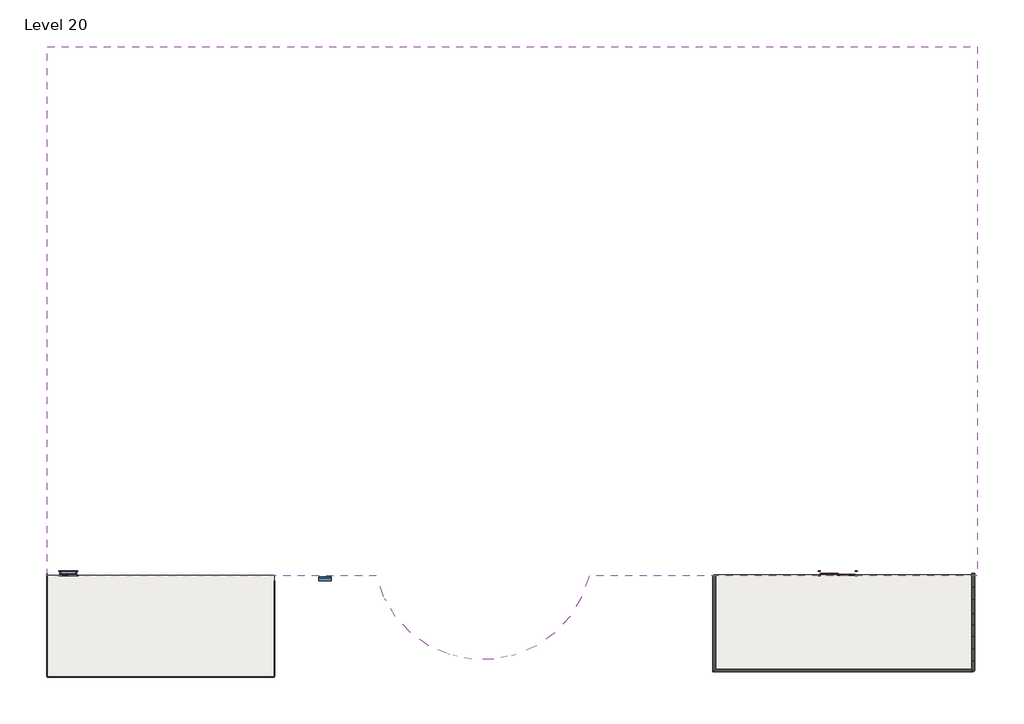
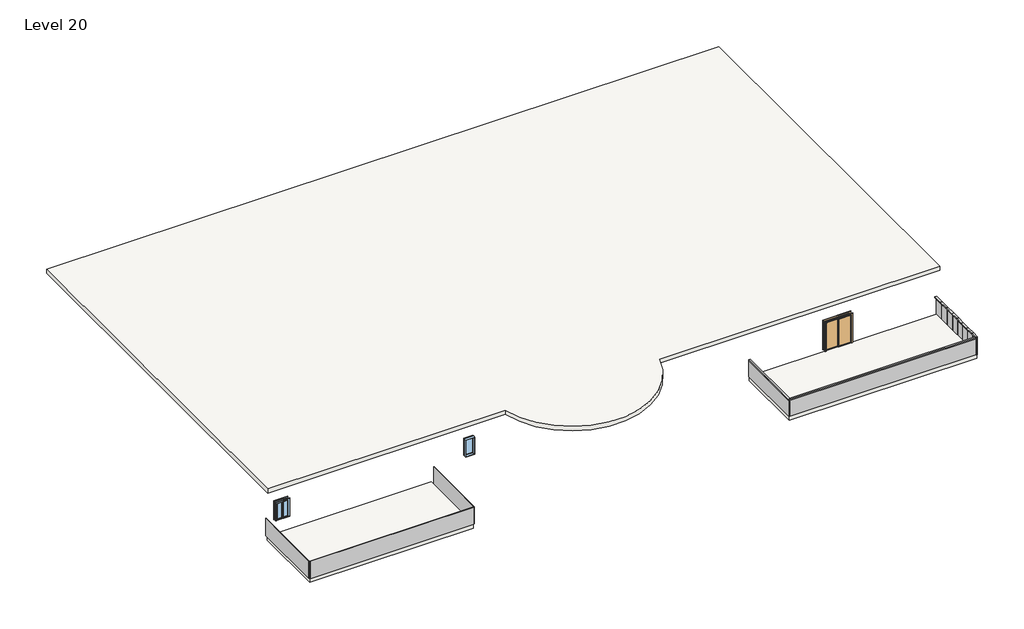
# One storey: 13 plates, 11 members, 3 slabs, 2 windows, 1 door.
"""IFC4 building model written with IfcOpenShell, lengths in millimetres."""

from ifc_helpers import new_model, si_unit, point, frame, frame_2d, origin, place, context, project, spatial, polyline, circle_curve, trimmed, segment, composite_curve, outline, extrude, transform, mapped, element, save
from components import door_076b30e0, member_75074519, member_47bfaf8a, member_50cacee6, member_623bfa76, member_1d9ef59f, member_15823cb3, member_bdd043b7, member_60525e8a, system_panel_glazed_689d74eb, system_panel_glazed_7af1c9c3, system_panel_glazed_b34e3459, system_panel_glazed_da164243, system_panel_glazed_d08d7fb2, system_panel_glazed_a18a7e0a, system_panel_glazed_d304929f, system_panel_glazed_b96adab1, system_panel_glazed_310057b8, system_panel_glazed_5fd648d4, window_bb17773d, window_80bd9af0

model = new_model("IFC4")

# Units and contexts
model_context = context("Model", 3, world=origin())
ifc_project = project(units=[si_unit("LENGTHUNIT", "METRE", prefix="MILLI")], contexts=[model_context])

# Site, building, storey
site = spatial("IfcSite", under=ifc_project)
building = spatial("IfcBuilding", under=site)
storey = spatial("IfcBuildingStorey", under=building, Name="Level 20", Elevation=33223.2)

# Door
placement = place(None, origin())
door_shape = door_076b30e0(model_context)
element("IfcDoor", 1, ObjectType="Door-Double-Sliding : 68\" x 80\"", at=placement, inside=storey, context=model_context, shape_type="MappedRepresentation", body=[
    mapped(door_shape, transform((18682.614721, -12227.7237084, 33223.2), x_axis=(-1.0, 0.0, 0.0), y_axis=(0.0, -1.0, 0.0), z_axis=(0.0, 0.0, 1.0))),
])

# Members
member_shape = member_75074519(model_context)
element("IfcMember", 2, ObjectType="Rectangular Mullion : 2.5\" x 5\" rectangular", at=placement, inside=storey, context=model_context, shape_type="MappedRepresentation", body=[
    mapped(member_shape, transform((25286.614721, -17100.0861335, 34442.4), x_axis=(1.0, 0.0, 0.0), y_axis=(0.0, 1.0, 0.0), z_axis=(0.0, 0.0, 1.0))),
])
member_2_shape = member_47bfaf8a(model_context)
element("IfcMember", 3, ObjectType="Rectangular Mullion : 2.5\" x 5\" rectangular", at=placement, inside=storey, context=model_context, shape_type="MappedRepresentation", body=[
    mapped(member_2_shape, transform((25286.614721, -16642.8861335, 34442.4), x_axis=(0.0, 0.0, 1.0), y_axis=(-1.0, 0.0, 0.0), z_axis=(0.0, -1.0, 0.0))),
])
member_3_shape = member_50cacee6(model_context)
element("IfcMember", 4, ObjectType="Rectangular Mullion : 2.5\" x 5\" rectangular", at=placement, inside=storey, context=model_context, shape_type="MappedRepresentation", body=[
    mapped(member_3_shape, transform((25286.614721, -15449.0861335, 34442.4), x_axis=(0.0, 0.0, 1.0), y_axis=(-1.0, 0.0, 0.0), z_axis=(0.0, -1.0, 0.0))),
])
member_4_shape = member_623bfa76(model_context)
element("IfcMember", 5, ObjectType="Rectangular Mullion : 2.5\" x 5\" rectangular", at=placement, inside=storey, context=model_context, shape_type="MappedRepresentation", body=[
    mapped(member_4_shape, transform((25286.614721, -14890.2861335, 34442.4), x_axis=(0.0, 0.0, 1.0), y_axis=(-1.0, 0.0, 0.0), z_axis=(0.0, -1.0, 0.0))),
])
element("IfcMember", 6, ObjectType="Rectangular Mullion : 2.5\" x 5\" rectangular", at=placement, inside=storey, context=model_context, shape_type="MappedRepresentation", body=[
    mapped(member_4_shape, transform((25286.614721, -16033.2861335, 34442.4), x_axis=(0.0, 0.0, 1.0), y_axis=(-1.0, 0.0, 0.0), z_axis=(0.0, -1.0, 0.0))),
])
member_5_shape = member_1d9ef59f(model_context)
element("IfcMember", 7, ObjectType="Rectangular Mullion : 2.5\" x 5\" rectangular", at=placement, inside=storey, context=model_context, shape_type="MappedRepresentation", body=[
    mapped(member_5_shape, transform((25286.614721, -13005.1778501, 34442.4), x_axis=(0.0, 0.0, 1.0), y_axis=(-1.0, 0.0, 0.0), z_axis=(0.0, -1.0, 0.0))),
])
element("IfcMember", 8, ObjectType="Rectangular Mullion : 2.5\" x 5\" rectangular", at=placement, inside=storey, context=model_context, shape_type="MappedRepresentation", body=[
    mapped(member_5_shape, transform((25286.614721, -13655.6319918, 34442.4), x_axis=(0.0, 0.0, 1.0), y_axis=(-1.0, 0.0, 0.0), z_axis=(0.0, -1.0, 0.0))),
])
element("IfcMember", 9, ObjectType="Rectangular Mullion : 2.5\" x 5\" rectangular", at=placement, inside=storey, context=model_context, shape_type="MappedRepresentation", body=[
    mapped(member_5_shape, transform((25286.614721, -14306.0861335, 34442.4), x_axis=(0.0, 0.0, 1.0), y_axis=(-1.0, 0.0, 0.0), z_axis=(0.0, -1.0, 0.0))),
])
member_6_shape = member_15823cb3(model_context)
element("IfcMember", 10, ObjectType="Rectangular Mullion : 2.5\" x 5\" rectangular", at=placement, inside=storey, context=model_context, shape_type="MappedRepresentation", body=[
    mapped(member_6_shape, transform((25286.614721, -17100.0861335, 34442.4), x_axis=(0.0, 0.0, 1.0), y_axis=(-1.0, 0.0, 0.0), z_axis=(0.0, -1.0, 0.0))),
])
member_7_shape = member_bdd043b7(model_context)
element("IfcMember", 11, ObjectType="Rectangular Mullion : 2.5\" x 5\" rectangular", at=placement, inside=storey, context=model_context, shape_type="MappedRepresentation", body=[
    mapped(member_7_shape, transform((12667.5594464, -12456.3237084, 34442.4), x_axis=(0.0, 0.0, 1.0), y_axis=(1.0, 0.0, 0.0), z_axis=(0.0, 1.0, 0.0))),
])
member_8_shape = member_60525e8a(model_context)
element("IfcMember", 12, ObjectType="Rectangular Mullion : 2.5\" x 5\" rectangular", at=placement, inside=storey, context=model_context, shape_type="MappedRepresentation", body=[
    mapped(member_8_shape, transform((12667.5594464, -17100.0861335, 34442.4), x_axis=(0.0, 0.0, 1.0), y_axis=(0.0, 1.0, 0.0), z_axis=(-1.0, 0.0, 0.0))),
])

# Plates
system_panel_glazed_shape = system_panel_glazed_689d74eb(model_context)
element("IfcPlate", 13, ObjectType="System Panel : Glazed", at=placement, inside=storey, context=model_context, shape_type="MappedRepresentation", body=[
    mapped(system_panel_glazed_shape, transform((18945.3370837, -17100.0861335, 33223.2), x_axis=(-1.0, 0.0, 0.0), y_axis=(0.0, -1.0, 0.0), z_axis=(0.0, 0.0, 1.0))),
])
system_panel_glazed_2_shape = system_panel_glazed_7af1c9c3(model_context)
element("IfcPlate", 14, ObjectType="System Panel : Glazed", at=placement, inside=storey, context=model_context, shape_type="MappedRepresentation", body=[
    mapped(system_panel_glazed_2_shape, transform((25286.614721, -16338.0861335, 33223.2), x_axis=(0.0, -1.0, 0.0), y_axis=(1.0, 0.0, 0.0), z_axis=(0.0, 0.0, 1.0))),
])
system_panel_glazed_3_shape = system_panel_glazed_b34e3459(model_context)
element("IfcPlate", 15, ObjectType="System Panel : Glazed", at=placement, inside=storey, context=model_context, shape_type="MappedRepresentation", body=[
    mapped(system_panel_glazed_3_shape, transform((25286.614721, -15169.6861335, 33223.2), x_axis=(0.0, -1.0, 0.0), y_axis=(1.0, 0.0, 0.0), z_axis=(0.0, 0.0, 1.0))),
])
system_panel_glazed_4_shape = system_panel_glazed_da164243(model_context)
element("IfcPlate", 16, ObjectType="System Panel : Glazed", at=placement, inside=storey, context=model_context, shape_type="MappedRepresentation", body=[
    mapped(system_panel_glazed_4_shape, transform((25286.614721, -15741.1861335, 33223.2), x_axis=(0.0, -1.0, 0.0), y_axis=(1.0, 0.0, 0.0), z_axis=(0.0, 0.0, 1.0))),
])
element("IfcPlate", 17, ObjectType="System Panel : Glazed", at=placement, inside=storey, context=model_context, shape_type="MappedRepresentation", body=[
    mapped(system_panel_glazed_4_shape, transform((25286.614721, -14598.1861335, 33223.2), x_axis=(0.0, -1.0, 0.0), y_axis=(1.0, 0.0, 0.0), z_axis=(0.0, 0.0, 1.0))),
])
system_panel_glazed_5_shape = system_panel_glazed_d08d7fb2(model_context)
element("IfcPlate", 18, ObjectType="System Panel : Glazed", at=placement, inside=storey, context=model_context, shape_type="MappedRepresentation", body=[
    mapped(system_panel_glazed_5_shape, transform((25286.614721, -12679.9507792, 33223.2), x_axis=(0.0, -1.0, 0.0), y_axis=(1.0, 0.0, 0.0), z_axis=(0.0, 0.0, 1.0))),
])
element("IfcPlate", 19, ObjectType="System Panel : Glazed", at=placement, inside=storey, context=model_context, shape_type="MappedRepresentation", body=[
    mapped(system_panel_glazed_5_shape, transform((25286.614721, -13980.8590627, 33223.2), x_axis=(0.0, -1.0, 0.0), y_axis=(1.0, 0.0, 0.0), z_axis=(0.0, 0.0, 1.0))),
])
element("IfcPlate", 20, ObjectType="System Panel : Glazed", at=placement, inside=storey, context=model_context, shape_type="MappedRepresentation", body=[
    mapped(system_panel_glazed_5_shape, transform((25286.614721, -13330.404921, 33223.2), x_axis=(0.0, -1.0, 0.0), y_axis=(1.0, 0.0, 0.0), z_axis=(0.0, 0.0, 1.0))),
])
system_panel_glazed_6_shape = system_panel_glazed_a18a7e0a(model_context)
element("IfcPlate", 21, ObjectType="System Panel : Glazed", at=placement, inside=storey, context=model_context, shape_type="MappedRepresentation", body=[
    mapped(system_panel_glazed_6_shape, transform((25286.614721, -16871.4861335, 33223.2), x_axis=(0.0, -1.0, 0.0), y_axis=(1.0, 0.0, 0.0), z_axis=(0.0, 0.0, 1.0))),
])
system_panel_glazed_7_shape = system_panel_glazed_d304929f(model_context)
element("IfcPlate", 22, ObjectType="System Panel : Glazed", at=placement, inside=storey, context=model_context, shape_type="MappedRepresentation", body=[
    mapped(system_panel_glazed_7_shape, transform((12667.5594464, -14778.204921, 33223.2), x_axis=(0.0, 1.0, 0.0), y_axis=(-1.0, 0.0, 0.0), z_axis=(0.0, 0.0, 1.0))),
])
system_panel_glazed_8_shape = system_panel_glazed_b96adab1(model_context)
element("IfcPlate", 23, ObjectType="System Panel : Glazed", at=placement, inside=storey, context=model_context, shape_type="MappedRepresentation", body=[
    mapped(system_panel_glazed_8_shape, transform((-14302.7926538, -17381.6656682, 33223.2), x_axis=(-1.0, 0.0, 0.0), y_axis=(0.0, -1.0, 0.0), z_axis=(0.0, 0.0, 1.0))),
])
system_panel_glazed_9_shape = system_panel_glazed_310057b8(model_context)
element("IfcPlate", 24, ObjectType="System Panel : Glazed", at=placement, inside=storey, context=model_context, shape_type="MappedRepresentation", body=[
    mapped(system_panel_glazed_9_shape, transform((-19823.785279, -14868.1946883, 33223.2), x_axis=(0.0, 1.0, 0.0), y_axis=(-1.0, 0.0, 0.0), z_axis=(0.0, 0.0, 1.0))),
])
system_panel_glazed_10_shape = system_panel_glazed_5fd648d4(model_context)
element("IfcPlate", 25, ObjectType="System Panel : Glazed", at=placement, inside=storey, context=model_context, shape_type="MappedRepresentation", body=[
    mapped(system_panel_glazed_10_shape, transform((-8781.8000285, -15050.2331996, 33223.2), x_axis=(0.0, -1.0, 0.0), y_axis=(1.0, 0.0, 0.0), z_axis=(0.0, 0.0, 1.0))),
])

# Slabs
element("IfcSlab", 26, ObjectType="Generic - 12\"", at=placement, inside=storey, context=model_context, shape_type="SweptSolid", body=[
    extrude(outline(composite_curve([segment(polyline([(25489.814721, 13330.837176), (25489.814721, -12475.562824), (6571.5594464, -12475.562824)]), True, "CONTINUOUS"), segment(trimmed(circle_curve(frame_2d((1385.214721, -11244.9297828)), 5330.3498284), [point((6571.5594464, -12475.562824))], [point((-3801.1300045, -12475.562824))], False, "CARTESIAN"), True, "CONTINUOUS"), segment(polyline([(-3801.1300045, -12475.562824), (-19823.785279, -12475.562824), (-19823.785279, 13330.837176), (25489.814721, 13330.837176)]), True, "CONTINUOUS")], self_intersect=False)), frame((0.0, 0.0, 36308.9464133), z_axis=(0.0, 0.0, 1.0), x_axis=(1.0, 0.0, 0.0)), (0.0, 0.0, 1.0), 304.8),
])
element("IfcSlab", 27, ObjectType="Generic - 12\"", at=placement, inside=storey, context=model_context, shape_type="SweptSolid", body=[
    extrude(outline(polyline([(25286.614721, -12426.4535448), (25286.614721, -17100.0861335), (12667.5594464, -17100.0861335), (12667.5594464, -12426.4535448), (25286.614721, -12426.4535448)])), frame((0.0, 0.0, 32918.4), z_axis=(0.0, 0.0, 1.0), x_axis=(1.0, 0.0, 0.0)), (0.0, 0.0, 1.0), 304.8),
])
element("IfcSlab", 28, ObjectType="Generic - 12\"", at=placement, inside=storey, context=model_context, shape_type="SweptSolid", body=[
    extrude(outline(polyline([(-8781.8000285, -12456.3237084), (-8781.8000285, -17381.6656682), (-19823.785279, -17381.6656682), (-19823.785279, -12456.3237084), (-8781.8000285, -12456.3237084)])), frame((0.0, 0.0, 32918.4), z_axis=(0.0, 0.0, 1.0), x_axis=(1.0, 0.0, 0.0)), (0.0, 0.0, 1.0), 304.8),
])

# Windows
window_shape = window_bb17773d(model_context)
element("IfcWindow", 29, ObjectType="Casement Dbl with Trim : 32\" x 48\"", at=placement, inside=storey, context=model_context, shape_type="MappedRepresentation", body=[
    mapped(window_shape, transform((-18807.785279, -12335.6737084, 33223.2), x_axis=(-1.0, 0.0, 0.0), y_axis=(0.0, -1.0, 0.0), z_axis=(0.0, 0.0, 1.0))),
])
window_2_shape = window_80bd9af0(model_context)
element("IfcWindow", 30, ObjectType="Fixed : 24\" x 48\"", at=placement, inside=storey, context=model_context, shape_type="MappedRepresentation", body=[
    mapped(window_2_shape, transform((-6272.885279, -12617.2007309, 33479.3632624), x_axis=(1.0, 0.0, 0.0), y_axis=(0.0, 1.0, 0.0), z_axis=(0.0, 0.0, 1.0))),
])

save(model, "model.ifc")

# Revit data of these elements
# Type "Door-Double-Sliding : 68\" x 80\""
#   Type Mark = "10"
#   Construction Type Id = "opn-d45"
#   Assembly Code = "C1020"
#   Analytic Construction = "Wood frame, double glass door "
#   Thickness = 0' - 2"
#   Thermal Resistance (R) = 1.8150 (h·ft²·°F)/BTU
#   Heat Transfer Coefficient (U) = 0.5510 BTU/(h·ft²·°F)
#   Height = 6' - 8"
#   Rail Width = 0' - 2"
#   Stiles = 0' - 2"
#   Trim Projection Ext = 0' - 1"
#   Trim Projection Int = 0' - 1"
#   Trim Width = 0' - 3"
#   Width = 5' - 8"
#   Define Thermal Properties by = 1
#   Glazing = Glass
#   Panel Material = Wood - Birch - Solid Stained Light Low Gloss
#   Trim Material = Paint - Sienna
#   Visual Light Transmittance = 0
#   Solar Heat Gain Coefficient = 0
#   Function = (empty or 0)
#   Wall Closure = (empty or 0)
# Type "Rectangular Mullion : 2.5\" x 5\" rectangular"
#   built-in parameter 1007304 = 0.416667 (stored number, unit not read)
#   built-in parameter 1007301 = 0.104167 (stored number, unit not read)
#   built-in parameter 1007300 = 0.104167 (stored number, unit not read)
# Type "System Panel : Glazed"
#   Construction Type Id = "GSP4R"
#   Analytic Construction = "1/8 in Pilkington single glazing"
#   Visual Light Transmittance = 0.9
#   Solar Heat Gain Coefficient = 0.86
#   Heat Transfer Coefficient (U) = 1.18115 BTU/(h·ft²·°F)
# Type "Generic - 12\""
#   Assembly Code = "B1010"
#   Function = 0
#   Layers, outside or top first: 1' - 0" no material (function 1)
# Type "Casement Dbl with Trim : 32\" x 48\""
#   Type Mark = "36"
#   Construction Type Id = "GSP4R"
#   Assembly Code = "B2020100"
#   Analytic Construction = "1/8 in Pilkington single glazing"
#   Visual Light Transmittance = 0.9
#   Solar Heat Gain Coefficient = 0.78
#   Heat Transfer Coefficient (U) = 0.6496 BTU/(h·ft²·°F)
#   Height = 4' - 0"
#   Default Sill Height = 3' - 0"
#   Trim Projection - Ext. = 0' - 0 1/2"
#   Trim Projection - Int. = 0' - 0 3/4"
#   Trim Width - Exterior = 0' - 3 1/2"
#   Trim Width - Interior = 0' - 3 1/2"
#   Width = 2' - 8"
#   Window Inset = 0' - 0 3/4"
#   Define Thermal Properties by = 1
#   Glass Pane Material = Glass
#   Sash Material = Sash
#   Trim Exterior Material = Trim
#   Trim Interior Material = Trim
#   Wall Closure = (empty or 0)
# Type "Fixed : 24\" x 48\""
#   Type Mark = "2"
#   Construction Type Id = "GSP4R"
#   Assembly Code = "B2020100"
#   Analytic Construction = "1/8 in Pilkington single glazing"
#   Visual Light Transmittance = 0.9
#   Solar Heat Gain Coefficient = 0.78
#   Heat Transfer Coefficient (U) = 0.6496 BTU/(h·ft²·°F)
#   Height = 4' - 0"
#   Default Sill Height = 3' - 0"
#   Width = 2' - 0"
#   Window Inset = 0' - 0 3/4"
#   Define Thermal Properties by = 1
#   Glass Pane Material = Glass
#   Sash Material = Sash
#   Wall Closure = (empty or 0)
# Element 1 (IfcDoor, "Door-Double-Sliding : 68\" x 80\"")
#   Phase Created = New Construction
#   Materials on its faces: "Paint - Sienna", "Wood - Birch - Solid Stained Light Low Gloss", "Glass"
# Elements 2, 3, 4, 5, 6, 7, 8, 9, 10, 11, 12 (IfcMember, "Rectangular Mullion : 2.5\" x 5\" rectangular")
#   Phase Created = New Construction
#   Materials on its faces: "Aluminum"
# Elements 13, 14, 15, 16, 17, 18, 19, 20, 21, 22, 23, 24, 25 (IfcPlate, "System Panel : Glazed")
#   Phase Created = New Construction
#   Materials on its faces: "Glass"
# Element 26 (IfcSlab, "Generic - 12\"")
#   Height Offset From Level = 11' - 1.48608"
#   Phase Created = New Construction
#   Materials on its faces: "Default Floor"
# Elements 27, 28 (IfcSlab, "Generic - 12\"")
#   Height Offset From Level = 0' - 0"
#   Phase Created = New Construction
#   Materials on its faces: "Default Floor"
# Element 29 (IfcWindow, "Casement Dbl with Trim : 32\" x 48\"")
#   Mark = "41"
#   Phase Created = New Construction
#   Materials on its faces: "Sash", "Trim", "Glass"
# Element 30 (IfcWindow, "Fixed : 24\" x 48\"")
#   Mark = "75"
#   Phase Created = New Construction
#   Materials on its faces: "Sash", "Glass"
# Materials
#   "Glass": class "Glass", colour RGB 0 128 192, transparency 0.75, Description = "Soda Lime Glass", Cost = 0
#   "Wood - Birch - Solid Stained Light Low Gloss": class "Wood", colour RGB 210 159 95, transparency 0, Cost = 0
#   "Paint - Sienna": colour RGB 118 70 51, transparency 0, Cost = 0
#   "Sash": class "Wood", colour RGB 224 178 126, transparency 0
#   "Trim": class "Wood", colour RGB 224 178 126, transparency 0
#   "Aluminum": class "Metal", colour RGB 247 247 247, transparency 0, Description = "Aluminum 6061", Cost = 0
#   "Default Floor": colour RGB 128 128 128, transparency 0
